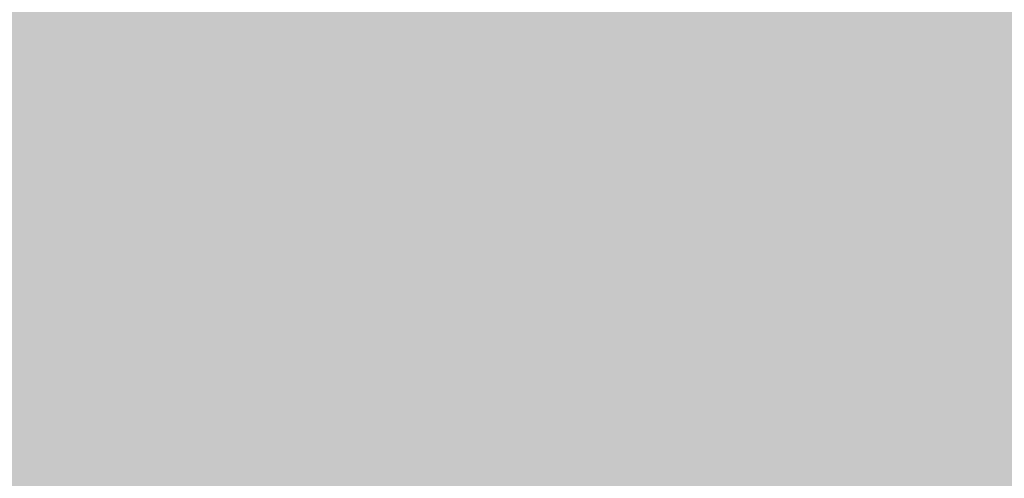
# Model space of a CAD drawing. Units: millimetres. Extents: x 0 to 2267, y 0 to 1823.
# Tile 139 of 256: x 1760 to 1802, y 1132 to 1152. Entities that reach past the tile are written whole.
import ezdxf

# ---------------------------------------------------------------- set-up
doc = ezdxf.new("R2010")
doc.units = ezdxf.units.MM
doc.header["$MEASUREMENT"] = 0
doc.layers.add('M-HATC', color=252, linetype='Continuous', lineweight=18)

msp = doc.modelspace()

# ---------------------------------------------------------------- hatches: boundary and pattern name
at = {"layer": 'M-HATC'}
h = msp.add_hatch(color=256, dxfattribs=at)
h.dxf.hatch_style = 1
h.paths.add_polyline_path([(2055.771, 1603.062), (1381.087, 1603.062), (1381.087, 1598.062), (2055.771, 1598.062)])
h.paths.add_polyline_path([(2055.771, 1598.062), (1381.087, 1598.062), (1381.087, 1593.062), (2055.771, 1593.062)])
h.paths.add_polyline_path([(2051.307, 1536.761), (1385.55, 1536.761), (1385.55, 1526.761), (1387.55, 1526.761), (1388.537, 1525.053), (1385.332, 1521.233), (1385.332, 1521.223), (2050.254, 1522.749), (2048.321, 1525.053), (2049.307, 1526.761), (2051.307, 1526.761)])
edge = h.paths.add_edge_path()
edge.add_arc((1847.535, 1379.149), 135, 222.60306, 222.89085, ccw=False)
edge.add_line((1748.166, 1287.766), (1683.092, 1287.766))
edge.add_arc((1583.724, 1379.149), 135, 317.10915, 317.39694, ccw=False)
edge.add_arc((1678.969, 1290.671), 5, 222.8909, 317.1091, ccw=False)
edge.add_arc((1774.213, 1379.149), 135, 222.60306, 222.89085, ccw=False)
edge.add_line((1674.845, 1287.766), (1609.771, 1287.766))
edge.add_arc((1510.403, 1379.149), 135, 317.10915, 317.39694, ccw=False)
edge.add_arc((1605.647, 1290.671), 5, 222.8909, 317.1091, ccw=False)
edge.add_arc((1700.892, 1379.149), 135, 222.60306, 222.89085, ccw=False)
edge.add_line((1601.524, 1287.766), (1536.45, 1287.766))
edge.add_arc((1437.081, 1379.149), 135, 317.10915, 317.39694, ccw=False)
edge.add_arc((1532.326, 1290.671), 5, 222.8909, 317.1091, ccw=False)
edge.add_arc((1627.571, 1379.149), 135, 222.60306, 222.89085, ccw=False)
edge.add_line((1528.203, 1287.766), (1505.929, 1287.766))
edge.add_spline(control_points=[(1505.929, 1287.766), (1504.262, 1287.766), (1504.262, 1282.766), (1505.929, 1282.766)], knot_values=[0, 0, 0, 0, 5, 5, 5, 5], degree=3, periodic=0)
edge.add_line((1505.929, 1282.766), (1930.929, 1282.766))
edge.add_spline(control_points=[(1930.929, 1282.766), (1932.596, 1282.766), (1932.596, 1287.766), (1930.929, 1287.766)], knot_values=[0, 0, 0, 0, 5, 5, 5, 5], degree=3, periodic=0)
edge.add_line((1930.929, 1287.766), (1903.056, 1287.766))
edge.add_arc((1803.688, 1379.149), 135, 317.10915, 317.39694, ccw=False)
edge.add_arc((1898.932, 1290.671), 5, 222.8909, 317.1091, ccw=False)
edge.add_arc((1994.177, 1379.149), 135, 222.60306, 222.89085, ccw=False)
edge.add_line((1894.809, 1287.766), (1829.735, 1287.766))
edge.add_arc((1730.366, 1379.149), 135, 317.10915, 317.39694, ccw=False)
edge.add_arc((1825.611, 1290.671), 5, 222.8909, 317.1091, ccw=False)
edge.add_arc((1920.856, 1379.149), 135, 222.60306, 222.89085, ccw=False)
edge.add_line((1821.487, 1287.766), (1756.413, 1287.766))
edge.add_arc((1657.045, 1379.149), 135, 317.10915, 317.39694, ccw=False)
edge.add_arc((1752.29, 1290.671), 5, 222.8909, 317.1091, ccw=False)
edge = h.paths.add_edge_path()
edge.add_spline(control_points=[(1843.429, 1227.247), (1845.096, 1227.247), (1845.096, 1232.247), (1843.429, 1232.247)], knot_values=[0, 0, 0, 0, 5, 5, 5, 5], degree=3, periodic=0)
edge.add_line((1843.429, 1232.247), (1593.429, 1232.247))
edge.add_spline(control_points=[(1593.429, 1232.247), (1591.762, 1232.247), (1591.762, 1227.247), (1593.429, 1227.247)], knot_values=[0, 0, 0, 0, 5, 5, 5, 5], degree=3, periodic=0)
edge.add_line((1593.429, 1227.247), (1843.429, 1227.247))
h.paths.add_polyline_path([(1905.929, 1127.417), (1530.929, 1127.417, 0.414214), (1520.929, 1117.417), (1530.929, 1117.417), (1915.929, 1117.417, 0.414214)])
edge = h.paths.add_edge_path()
edge.add_arc((1397.086, 1498.408), 12.73, 90.7821, 190.8787, ccw=False)
edge.add_line((1396.912, 1511.136), (1428.01, 1511.349))
edge.add_line((1428.01, 1511.349), (1433.01, 1511.349))
edge.add_line((1433.01, 1511.349), (1434.439, 1511.349))
edge.add_arc((1419.474, 1498.08), 20, 41.561, 74.0821)
edge.add_line((1424.959, 1517.314), (1399.935, 1517.256))
edge.add_spline(control_points=[(1399.931, 1517.256), (1399.884, 1517.213), (1399.833, 1517.169), (1399.777, 1517.124)], knot_values=[11.567499, 11.567499, 11.567499, 11.567499, 11.814249, 11.814249, 11.814249, 11.814249], degree=3, periodic=0)
edge.add_spline(control_points=[(1399.633, 1517.01), (1399.583, 1516.972), (1399.531, 1516.934), (1399.476, 1516.895)], knot_values=[11.167718, 11.167718, 11.167718, 11.167718, 11.365188, 11.365188, 11.365188, 11.365188], degree=3, periodic=0)
edge.add_spline(control_points=[(1399.34, 1516.8), (1399.151, 1516.672), (1398.938, 1516.538), (1398.704, 1516.399)], knot_values=[10.376405, 10.376405, 10.376405, 10.376405, 11.00994, 11.00994, 11.00994, 11.00994], degree=3, periodic=0)
edge.add_spline(control_points=[(1398.657, 1516.372), (1398.579, 1516.326), (1398.498, 1516.28), (1398.415, 1516.233)], knot_values=[10.125175, 10.125175, 10.125175, 10.125175, 10.334406, 10.334406, 10.334406, 10.334406], degree=3, periodic=0)
edge.add_spline(control_points=[(1398.264, 1516.149), (1398.196, 1516.111), (1398.126, 1516.073), (1398.055, 1516.035)], knot_values=[9.832246, 9.832246, 9.832246, 9.832246, 9.999658, 9.999658, 9.999658, 9.999658], degree=3, periodic=0)
edge.add_spline(control_points=[(1397.999, 1516.005), (1397.731, 1515.862), (1397.446, 1515.717), (1397.147, 1515.571)], knot_values=[9.161808, 9.161808, 9.161808, 9.161808, 9.787769, 9.787769, 9.787769, 9.787769], degree=3, periodic=0)
edge.add_spline(control_points=[(1397.147, 1515.571), (1396.842, 1515.423), (1396.522, 1515.274), (1396.191, 1515.126)], knot_values=[8.524455, 8.524455, 8.524455, 8.524455, 9.161808, 9.161808, 9.161808, 9.161808], degree=3, periodic=0)
edge.add_spline(control_points=[(1396.078, 1515.076), (1395.985, 1515.035), (1395.892, 1514.994), (1395.798, 1514.953)], knot_values=[8.275193, 8.275193, 8.275193, 8.275193, 8.451726, 8.451726, 8.451726, 8.451726], degree=3, periodic=0)
edge.add_spline(control_points=[(1395.602, 1514.869), (1395.5, 1514.826), (1395.397, 1514.782), (1395.293, 1514.739)], knot_values=[7.962917, 7.962917, 7.962917, 7.962917, 8.152764, 8.152764, 8.152764, 8.152764], degree=3, periodic=0)
edge.add_spline(control_points=[(1395.212, 1514.706), (1394.828, 1514.547), (1394.435, 1514.393), (1394.036, 1514.244)], knot_values=[7.21254, 7.21254, 7.21254, 7.21254, 7.913148, 7.913148, 7.913148, 7.913148], degree=3, periodic=0)
edge.add_spline(control_points=[(1394.036, 1514.244), (1393.708, 1514.121), (1393.375, 1514.003), (1393.043, 1513.889)], knot_values=[6.633733, 6.633733, 6.633733, 6.633733, 7.21254, 7.21254, 7.21254, 7.21254], degree=3, periodic=0)
edge.add_spline(control_points=[(1392.821, 1513.815), (1392.72, 1513.781), (1392.618, 1513.748), (1392.517, 1513.715)], knot_values=[6.328796, 6.328796, 6.328796, 6.328796, 6.505493, 6.505493, 6.505493, 6.505493], degree=3, periodic=0)
edge.add_spline(control_points=[(1392.517, 1513.715), (1392.319, 1513.652), (1392.121, 1513.59), (1391.924, 1513.531)], knot_values=[5.984605, 5.984605, 5.984605, 5.984605, 6.328796, 6.328796, 6.328796, 6.328796], degree=3, periodic=0)
edge.add_spline(control_points=[(1391.792, 1513.491), (1391.312, 1513.35), (1390.838, 1513.224), (1390.378, 1513.117)], knot_values=[5.066697, 5.066697, 5.066697, 5.066697, 5.907055, 5.907055, 5.907055, 5.907055], degree=3, periodic=0)
edge.add_spline(control_points=[(1390.378, 1513.117), (1390.18, 1513.071), (1389.984, 1513.028), (1389.791, 1512.99)], knot_values=[4.70367, 4.70367, 4.70367, 4.70367, 5.066695, 5.066695, 5.066695, 5.066695], degree=3, periodic=0)
edge.add_spline(control_points=[(1389.422, 1512.92), (1389.246, 1512.889), (1389.073, 1512.862), (1388.904, 1512.838)], knot_values=[4.130571, 4.130571, 4.130571, 4.130571, 4.469816, 4.469816, 4.469816, 4.469816], degree=3, periodic=0)
edge.add_spline(control_points=[(1388.904, 1512.838), (1388.591, 1512.795), (1388.291, 1512.764), (1388.007, 1512.749)], knot_values=[3.504031, 3.504031, 3.504031, 3.504031, 4.130571, 4.130571, 4.130571, 4.130571], degree=3, periodic=0)
edge.add_spline(control_points=[(1387.936, 1512.746), (1387.854, 1512.742), (1387.773, 1512.74), (1387.694, 1512.739)], knot_values=[3.268866, 3.268866, 3.268866, 3.268866, 3.451164, 3.451164, 3.451164, 3.451164], degree=3, periodic=0)
edge.add_spline(control_points=[(1387.335, 1512.744), (1387.208, 1512.75), (1387.085, 1512.76), (1386.967, 1512.774)], knot_values=[2.670686, 2.670686, 2.670686, 2.670686, 2.984, 2.984, 2.984, 2.984], degree=3, periodic=0)
edge.add_spline(control_points=[(1386.833, 1512.792), (1386.821, 1512.794), (1386.809, 1512.796), (1386.797, 1512.798)], knot_values=[2.516981, 2.516981, 2.516981, 2.516981, 2.549528, 2.549528, 2.549528, 2.549528], degree=3, periodic=0)
edge.add_spline(control_points=[(1386.453, 1512.873), (1386.426, 1512.881), (1386.399, 1512.889), (1386.373, 1512.897)], knot_values=[2.095869, 2.095869, 2.095869, 2.095869, 2.17941, 2.17941, 2.17941, 2.17941], degree=3, periodic=0)
edge.add_spline(control_points=[(1386.069, 1513.019), (1386.063, 1513.022), (1386.058, 1513.025), (1386.052, 1513.028)], knot_values=[1.72453, 1.72453, 1.72453, 1.72453, 1.745933, 1.745933, 1.745933, 1.745933], degree=3, periodic=0)
edge.add_arc((1399.474, 1498.08), 20, 131.8243, 180)
edge.add_arc((1630.334, 1505.548), 250.971, 181.70518, 236.42798)
edge.add_arc((1605.34, 1483.304), 218.782, 238.66083, 243.34961)
edge.add_arc((1647.091, 1510.359), 262.899, 183.12984, 237.85344, ccw=False)
h.paths.add_polyline_path([(1406.537, 1391.964, 0.149382), (1491.551, 1296.442, -0.129517)], flags=17)
edge = h.paths.add_edge_path()
edge.add_arc((2037.384, 1498.08), 20, 0, 48.2659)
edge.add_spline(control_points=[(2050.697, 1513.005), (2050.651, 1512.985), (2050.603, 1512.966), (2050.554, 1512.948)], knot_values=[1.835652, 1.835652, 1.835652, 1.835652, 2.000781, 2.000781, 2.000781, 2.000781], degree=3, periodic=0)
edge.add_spline(control_points=[(2050.462, 1512.917), (2050.479, 1512.922), (2050.496, 1512.928), (2050.513, 1512.934)], knot_values=[2.045477, 2.045477, 2.045477, 2.045477, 2.101389, 2.101389, 2.101389, 2.101389], degree=3, periodic=0)
edge.add_spline(control_points=[(2050.129, 1512.834), (2050.198, 1512.847), (2050.266, 1512.862), (2050.331, 1512.879)], knot_values=[2.237629, 2.237629, 2.237629, 2.237629, 2.435841, 2.435841, 2.435841, 2.435841], degree=3, periodic=0)
edge.add_spline(control_points=[(2050.095, 1512.828), (2050.106, 1512.83), (2050.118, 1512.832), (2050.129, 1512.834)], knot_values=[2.435841, 2.435841, 2.435841, 2.435841, 2.468321, 2.468321, 2.468321, 2.468321], degree=3, periodic=0)
edge.add_spline(control_points=[(2049.784, 1512.785), (2049.855, 1512.792), (2049.924, 1512.801), (2049.992, 1512.811)], knot_values=[2.563852, 2.563852, 2.563852, 2.563852, 2.748541, 2.748541, 2.748541, 2.748541], degree=3, periodic=0)
edge.add_spline(control_points=[(2049.405, 1512.762), (2049.536, 1512.765), (2049.663, 1512.773), (2049.784, 1512.785)], knot_values=[2.748541, 2.748541, 2.748541, 2.748541, 3.064882, 3.064882, 3.064882, 3.064882], degree=3, periodic=0)
edge.add_spline(control_points=[(2049.17, 1512.76), (2049.234, 1512.759), (2049.297, 1512.759), (2049.358, 1512.761)], knot_values=[3.102309, 3.102309, 3.102309, 3.102309, 3.2503, 3.2503, 3.2503, 3.2503], degree=3, periodic=0)
edge.add_spline(control_points=[(2048.857, 1512.769), (2048.964, 1512.764), (2049.068, 1512.761), (2049.17, 1512.76)], knot_values=[3.2503, 3.2503, 3.2503, 3.2503, 3.486069, 3.486069, 3.486069, 3.486069], degree=3, periodic=0)
edge.add_spline(control_points=[(2048.692, 1512.779), (2048.373, 1512.801), (2048.035, 1512.841), (2047.682, 1512.897)], knot_values=[3.606429, 3.606429, 3.606429, 3.606429, 4.2989, 4.2989, 4.2989, 4.2989], degree=3, periodic=0)
edge.add_spline(control_points=[(2047.682, 1512.897), (2047.546, 1512.919), (2047.408, 1512.942), (2047.268, 1512.969)], knot_values=[4.2989, 4.2989, 4.2989, 4.2989, 4.565769, 4.565769, 4.565769, 4.565769], degree=3, periodic=0)
edge.add_spline(control_points=[(2047.268, 1512.969), (2047.145, 1512.991), (2047.021, 1513.016), (2046.895, 1513.042)], knot_values=[4.565769, 4.565769, 4.565769, 4.565769, 4.799971, 4.799971, 4.799971, 4.799971], degree=3, periodic=0)
edge.add_spline(control_points=[(2046.895, 1513.042), (2046.529, 1513.119), (2046.151, 1513.209), (2045.768, 1513.311)], knot_values=[4.799971, 4.799971, 4.799971, 4.799971, 5.483718, 5.483718, 5.483718, 5.483718], degree=3, periodic=0)
edge.add_spline(control_points=[(2045.768, 1513.311), (2045.372, 1513.415), (2044.97, 1513.532), (2044.566, 1513.659)], knot_values=[5.483718, 5.483718, 5.483718, 5.483718, 6.187866, 6.187866, 6.187866, 6.187866], degree=3, periodic=0)
edge.add_spline(control_points=[(2044.566, 1513.659), (2044.415, 1513.706), (2044.263, 1513.755), (2044.112, 1513.805)], knot_values=[6.187866, 6.187866, 6.187866, 6.187866, 6.451551, 6.451551, 6.451551, 6.451551], degree=3, periodic=0)
edge.add_spline(control_points=[(2044.112, 1513.805), (2043.997, 1513.843), (2043.882, 1513.881), (2043.767, 1513.92)], knot_values=[6.451551, 6.451551, 6.451551, 6.451551, 6.651434, 6.651434, 6.651434, 6.651434], degree=3, periodic=0)
edge.add_spline(control_points=[(2043.767, 1513.92), (2043.372, 1514.055), (2042.977, 1514.198), (2042.589, 1514.346)], knot_values=[6.651434, 6.651434, 6.651434, 6.651434, 7.338879, 7.338879, 7.338879, 7.338879], degree=3, periodic=0)
edge.add_spline(control_points=[(2042.589, 1514.346), (2042.164, 1514.507), (2041.746, 1514.675), (2041.341, 1514.846)], knot_values=[7.338879, 7.338879, 7.338879, 7.338879, 8.089209, 8.089209, 8.089209, 8.089209], degree=3, periodic=0)
edge.add_spline(control_points=[(2041.341, 1514.846), (2041.103, 1514.946), (2040.869, 1515.048), (2040.64, 1515.15)], knot_values=[8.089209, 8.089209, 8.089209, 8.089209, 8.529587, 8.529587, 8.529587, 8.529587], degree=3, periodic=0)
edge.add_spline(control_points=[(2040.51, 1515.209), (2040.082, 1515.402), (2039.675, 1515.597), (2039.295, 1515.789)], knot_values=[8.613818, 8.613818, 8.613818, 8.613818, 9.44571, 9.44571, 9.44571, 9.44571], degree=3, periodic=0)
edge.add_spline(control_points=[(2039.295, 1515.789), (2039.062, 1515.907), (2038.839, 1516.025), (2038.629, 1516.14)], knot_values=[9.44571, 9.44571, 9.44571, 9.44571, 9.956404, 9.956404, 9.956404, 9.956404], degree=3, periodic=0)
edge.add_spline(control_points=[(2038.629, 1516.14), (2038.519, 1516.2), (2038.412, 1516.26), (2038.309, 1516.319)], knot_values=[9.956404, 9.956404, 9.956404, 9.956404, 10.223542, 10.223542, 10.223542, 10.223542], degree=3, periodic=0)
edge.add_spline(control_points=[(2038.309, 1516.319), (2038.214, 1516.374), (2038.122, 1516.428), (2038.033, 1516.481)], knot_values=[10.223542, 10.223542, 10.223542, 10.223542, 10.47051, 10.47051, 10.47051, 10.47051], degree=3, periodic=0)
edge.add_spline(control_points=[(2038.033, 1516.481), (2037.786, 1516.63), (2037.564, 1516.773), (2037.372, 1516.909)], knot_values=[10.47051, 10.47051, 10.47051, 10.47051, 11.15767, 11.15767, 11.15767, 11.15767], degree=3, periodic=0)
edge.add_spline(control_points=[(2037.372, 1516.909), (2037.279, 1516.975), (2037.193, 1517.04), (2037.114, 1517.102)], knot_values=[11.15767, 11.15767, 11.15767, 11.15767, 11.49227, 11.49227, 11.49227, 11.49227], degree=3, periodic=0)
edge.add_spline(control_points=[(2036.856, 1517.326), (2036.915, 1517.269), (2036.981, 1517.21), (2037.056, 1517.149)], knot_values=[11.577341, 11.577341, 11.577341, 11.577341, 11.91035, 11.91035, 11.91035, 11.91035], degree=3, periodic=0)
edge.add_spline(control_points=[(2036.807, 1517.375), (2036.823, 1517.359), (2036.839, 1517.342), (2036.856, 1517.326)], knot_values=[11.91035, 11.91035, 11.91035, 11.91035, 12.007402, 12.007402, 12.007402, 12.007402], degree=3, periodic=0)
edge.add_spline(control_points=[(2036.702, 1517.494), (2036.71, 1517.483), (2036.72, 1517.472), (2036.729, 1517.461)], knot_values=[12.184155, 12.184155, 12.184155, 12.184155, 12.255409, 12.255409, 12.255409, 12.255409], degree=3, periodic=0)
edge.add_spline(control_points=[(2036.616, 1517.621), (2036.62, 1517.613), (2036.624, 1517.606), (2036.629, 1517.598)], knot_values=[12.487913, 12.487913, 12.487913, 12.487913, 12.541035, 12.541035, 12.541035, 12.541035], degree=3, periodic=0)
edge.add_spline(control_points=[(2036.563, 1517.786), (2036.564, 1517.779), (2036.564, 1517.773), (2036.565, 1517.766)], knot_values=[12.911761, 12.911761, 12.911761, 12.911761, 12.968286, 12.968286, 12.968286, 12.968286], degree=3, periodic=0)
edge.add_spline(control_points=[(2036.617, 1517.93), (2036.612, 1517.926), (2036.609, 1517.921), (2036.605, 1517.916)], knot_values=[13.382527, 13.382527, 13.382527, 13.382527, 13.433791, 13.433791, 13.433791, 13.433791], degree=3, periodic=0)
edge.add_spline(control_points=[(2036.749, 1518.017), (2036.736, 1518.012), (2036.724, 1518.006), (2036.712, 1518)], knot_values=[13.726299, 13.726299, 13.726299, 13.726299, 13.809928, 13.809928, 13.809928, 13.809928], degree=3, periodic=0)
edge.add_spline(control_points=[(2036.86, 1518.053), (2036.839, 1518.047), (2036.818, 1518.042), (2036.799, 1518.035)], knot_values=[13.910887, 13.910887, 13.910887, 13.910887, 14.02153, 14.02153, 14.02153, 14.02153], degree=3, periodic=0)
edge.add_line((2036.964, 1518.08), (2032.384, 1518.08))
edge.add_line((2032.384, 1518.08), (2027.384, 1518.08))
edge.add_line((2027.384, 1518.08), (2022.384, 1518.08))
edge.add_line((2022.384, 1518.08), (2017.384, 1518.08))
edge.add_arc((2017.384, 1498.08), 20, 90, 138.439)
edge.add_line((2002.419, 1511.349), (2003.848, 1511.349))
edge.add_line((2003.848, 1511.349), (2008.848, 1511.349))
edge.add_line((2008.848, 1511.349), (2039.772, 1511.138))
edge.add_arc((2039.772, 1498.408), 12.73, -10.8787, 90, ccw=False)
edge.add_arc((1789.767, 1510.359), 262.899, 302.14656, 356.87016, ccw=False)
edge.add_arc((1831.518, 1483.304), 218.782, 296.65039, 301.33917)
edge.add_arc((1806.524, 1505.548), 250.971, 303.57202, 358.29482)
h.paths.add_polyline_path([(2030.321, 1391.964, -0.129517), (1945.307, 1296.442, 0.149382)], flags=17)
edge = h.paths.add_edge_path()
edge.add_spline(control_points=[(2037.246, 1518.082), (2037.29, 1518.081), (2037.336, 1518.08), (2037.384, 1518.08)], knot_values=[0.000012, 0.000012, 0.000012, 0.000012, 0.144754, 0.144754, 0.144754, 0.144754], degree=3, periodic=0)
edge.add_line((2037.336, 1518.08), (2037.01, 1518.08))
edge.add_spline(control_points=[(2037.01, 1518.08), (2036.982, 1518.077), (2036.956, 1518.073), (2036.931, 1518.068)], knot_values=[14.13465, 14.13465, 14.13465, 14.13465, 14.247197, 14.247197, 14.247197, 14.247197], degree=3, periodic=0)
edge.add_spline(control_points=[(2036.931, 1518.068), (2036.928, 1518.067), (2036.924, 1518.067), (2036.921, 1518.066)], knot_values=[14.118315, 14.118315, 14.118315, 14.118315, 14.13465, 14.13465, 14.13465, 14.13465], degree=3, periodic=0)
edge.add_spline(control_points=[(2036.921, 1518.066), (2036.912, 1518.064), (2036.903, 1518.063), (2036.895, 1518.061)], knot_values=[14.078086, 14.078086, 14.078086, 14.078086, 14.118315, 14.118315, 14.118315, 14.118315], degree=3, periodic=0)
edge.add_spline(control_points=[(2036.895, 1518.061), (2036.883, 1518.058), (2036.872, 1518.056), (2036.86, 1518.053)], knot_values=[14.02153, 14.02153, 14.02153, 14.02153, 14.078086, 14.078086, 14.078086, 14.078086], degree=3, periodic=0)
edge.add_spline(control_points=[(2036.86, 1518.053), (2036.839, 1518.047), (2036.818, 1518.042), (2036.799, 1518.035)], knot_values=[13.910887, 13.910887, 13.910887, 13.910887, 14.02153, 14.02153, 14.02153, 14.02153], degree=3, periodic=0)
edge.add_spline(control_points=[(2036.799, 1518.035), (2036.798, 1518.035), (2036.797, 1518.035), (2036.797, 1518.035)], knot_values=[13.906906, 13.906906, 13.906906, 13.906906, 13.910887, 13.910887, 13.910887, 13.910887], degree=3, periodic=0)
edge.add_spline(control_points=[(2036.797, 1518.035), (2036.788, 1518.032), (2036.78, 1518.029), (2036.772, 1518.026)], knot_values=[13.857826, 13.857826, 13.857826, 13.857826, 13.906906, 13.906906, 13.906906, 13.906906], degree=3, periodic=0)
edge.add_spline(control_points=[(2036.772, 1518.026), (2036.764, 1518.023), (2036.756, 1518.02), (2036.749, 1518.017)], knot_values=[13.809928, 13.809928, 13.809928, 13.809928, 13.857826, 13.857826, 13.857826, 13.857826], degree=3, periodic=0)
edge.add_spline(control_points=[(2036.749, 1518.017), (2036.736, 1518.012), (2036.724, 1518.006), (2036.712, 1518)], knot_values=[13.726299, 13.726299, 13.726299, 13.726299, 13.809928, 13.809928, 13.809928, 13.809928], degree=3, periodic=0)
edge.add_spline(control_points=[(2036.712, 1518), (2036.712, 1518), (2036.712, 1518), (2036.711, 1518)], knot_values=[13.723993, 13.723993, 13.723993, 13.723993, 13.726299, 13.726299, 13.726299, 13.726299], degree=3, periodic=0)
edge.add_spline(control_points=[(2036.711, 1518), (2036.706, 1517.997), (2036.701, 1517.994), (2036.696, 1517.992)], knot_values=[13.686536, 13.686536, 13.686536, 13.686536, 13.723993, 13.723993, 13.723993, 13.723993], degree=3, periodic=0)
edge.add_spline(control_points=[(2036.696, 1517.992), (2036.692, 1517.989), (2036.687, 1517.987), (2036.683, 1517.984)], knot_values=[13.651251, 13.651251, 13.651251, 13.651251, 13.686536, 13.686536, 13.686536, 13.686536], degree=3, periodic=0)
edge.add_spline(control_points=[(2036.683, 1517.984), (2036.676, 1517.98), (2036.67, 1517.976), (2036.664, 1517.971)], knot_values=[13.596804, 13.596804, 13.596804, 13.596804, 13.651251, 13.651251, 13.651251, 13.651251], degree=3, periodic=0)
edge.add_spline(control_points=[(2036.664, 1517.971), (2036.664, 1517.971), (2036.663, 1517.971), (2036.663, 1517.971)], knot_values=[13.593956, 13.593956, 13.593956, 13.593956, 13.596804, 13.596804, 13.596804, 13.596804], degree=3, periodic=0)
edge.add_spline(control_points=[(2036.663, 1517.971), (2036.66, 1517.969), (2036.658, 1517.967), (2036.655, 1517.965)], knot_values=[13.570322, 13.570322, 13.570322, 13.570322, 13.593956, 13.593956, 13.593956, 13.593956], degree=3, periodic=0)
edge.add_spline(control_points=[(2036.655, 1517.965), (2036.653, 1517.963), (2036.65, 1517.961), (2036.647, 1517.959)], knot_values=[13.545477, 13.545477, 13.545477, 13.545477, 13.570322, 13.570322, 13.570322, 13.570322], degree=3, periodic=0)
edge.add_spline(control_points=[(2036.647, 1517.959), (2036.647, 1517.959), (2036.647, 1517.959), (2036.647, 1517.959)], knot_values=[13.543931, 13.543931, 13.543931, 13.543931, 13.545477, 13.545477, 13.545477, 13.545477], degree=3, periodic=0)
edge.add_spline(control_points=[(2036.647, 1517.959), (2036.641, 1517.954), (2036.636, 1517.949), (2036.631, 1517.945)], knot_values=[13.488237, 13.488237, 13.488237, 13.488237, 13.543931, 13.543931, 13.543931, 13.543931], degree=3, periodic=0)
edge.add_spline(control_points=[(2036.631, 1517.945), (2036.628, 1517.942), (2036.626, 1517.94), (2036.623, 1517.937)], knot_values=[13.460307, 13.460307, 13.460307, 13.460307, 13.488237, 13.488237, 13.488237, 13.488237], degree=3, periodic=0)
edge.add_spline(control_points=[(2036.623, 1517.937), (2036.622, 1517.936), (2036.62, 1517.934), (2036.618, 1517.932)], knot_values=[13.439712, 13.439712, 13.439712, 13.439712, 13.460307, 13.460307, 13.460307, 13.460307], degree=3, periodic=0)
edge.add_spline(control_points=[(2036.618, 1517.932), (2036.618, 1517.931), (2036.617, 1517.931), (2036.617, 1517.93)], knot_values=[13.433791, 13.433791, 13.433791, 13.433791, 13.439712, 13.439712, 13.439712, 13.439712], degree=3, periodic=0)
edge.add_spline(control_points=[(2036.617, 1517.93), (2036.612, 1517.926), (2036.609, 1517.921), (2036.605, 1517.916)], knot_values=[13.382527, 13.382527, 13.382527, 13.382527, 13.433791, 13.433791, 13.433791, 13.433791], degree=3, periodic=0)
edge.add_spline(control_points=[(2036.605, 1517.916), (2036.603, 1517.913), (2036.6, 1517.91), (2036.598, 1517.907)], knot_values=[13.350017, 13.350017, 13.350017, 13.350017, 13.382527, 13.382527, 13.382527, 13.382527], degree=3, periodic=0)
edge.add_spline(control_points=[(2036.598, 1517.907), (2036.597, 1517.906), (2036.596, 1517.904), (2036.595, 1517.903)], knot_values=[13.333922, 13.333922, 13.333922, 13.333922, 13.350017, 13.350017, 13.350017, 13.350017], degree=3, periodic=0)
edge.add_spline(control_points=[(2036.595, 1517.903), (2036.595, 1517.902), (2036.594, 1517.901), (2036.593, 1517.9)], knot_values=[13.323828, 13.323828, 13.323828, 13.323828, 13.333922, 13.333922, 13.333922, 13.333922], degree=3, periodic=0)
edge.add_spline(control_points=[(2036.593, 1517.9), (2036.59, 1517.895), (2036.588, 1517.891), (2036.585, 1517.886)], knot_values=[13.277545, 13.277545, 13.277545, 13.277545, 13.323828, 13.323828, 13.323828, 13.323828], degree=3, periodic=0)
edge.add_spline(control_points=[(2036.585, 1517.886), (2036.584, 1517.883), (2036.582, 1517.879), (2036.58, 1517.875)], knot_values=[13.240119, 13.240119, 13.240119, 13.240119, 13.277545, 13.277545, 13.277545, 13.277545], degree=3, periodic=0)
edge.add_spline(control_points=[(2036.58, 1517.875), (2036.58, 1517.874), (2036.579, 1517.873), (2036.578, 1517.872)], knot_values=[13.228211, 13.228211, 13.228211, 13.228211, 13.240119, 13.240119, 13.240119, 13.240119], degree=3, periodic=0)
edge.add_spline(control_points=[(2036.578, 1517.872), (2036.578, 1517.87), (2036.577, 1517.869), (2036.577, 1517.868)], knot_values=[13.215717, 13.215717, 13.215717, 13.215717, 13.228211, 13.228211, 13.228211, 13.228211], degree=3, periodic=0)
edge.add_spline(control_points=[(2036.577, 1517.868), (2036.575, 1517.864), (2036.574, 1517.86), (2036.573, 1517.857)], knot_values=[13.179847, 13.179847, 13.179847, 13.179847, 13.215717, 13.215717, 13.215717, 13.215717], degree=3, periodic=0)
edge.add_spline(control_points=[(2036.573, 1517.857), (2036.571, 1517.851), (2036.57, 1517.846), (2036.569, 1517.841)], knot_values=[13.132017, 13.132017, 13.132017, 13.132017, 13.179847, 13.179847, 13.179847, 13.179847], degree=3, periodic=0)
edge.add_spline(control_points=[(2036.569, 1517.841), (2036.568, 1517.84), (2036.568, 1517.839), (2036.568, 1517.838)], knot_values=[13.122482, 13.122482, 13.122482, 13.122482, 13.132017, 13.132017, 13.132017, 13.132017], degree=3, periodic=0)
edge.add_spline(control_points=[(2036.568, 1517.838), (2036.568, 1517.836), (2036.567, 1517.835), (2036.567, 1517.833)], knot_values=[13.105592, 13.105592, 13.105592, 13.105592, 13.122482, 13.122482, 13.122482, 13.122482], degree=3, periodic=0)
edge.add_spline(control_points=[(2036.567, 1517.833), (2036.566, 1517.829), (2036.566, 1517.826), (2036.565, 1517.822)], knot_values=[13.074063, 13.074063, 13.074063, 13.074063, 13.105592, 13.105592, 13.105592, 13.105592], degree=3, periodic=0)
edge.add_spline(control_points=[(2036.565, 1517.822), (2036.565, 1517.822), (2036.565, 1517.822), (2036.565, 1517.822)], knot_values=[13.074043, 13.074043, 13.074043, 13.074043, 13.074063, 13.074063, 13.074063, 13.074063], degree=3, periodic=0)
edge.add_spline(control_points=[(2036.565, 1517.822), (2036.564, 1517.816), (2036.564, 1517.811), (2036.564, 1517.805)], knot_values=[13.021884, 13.021884, 13.021884, 13.021884, 13.074043, 13.074043, 13.074043, 13.074043], degree=3, periodic=0)
edge.add_spline(control_points=[(2036.564, 1517.805), (2036.564, 1517.804), (2036.564, 1517.803), (2036.564, 1517.803)], knot_values=[13.01674, 13.01674, 13.01674, 13.01674, 13.021884, 13.021884, 13.021884, 13.021884], degree=3, periodic=0)
edge.add_spline(control_points=[(2036.564, 1517.803), (2036.563, 1517.801), (2036.563, 1517.798), (2036.563, 1517.796)], knot_values=[12.996438, 12.996438, 12.996438, 12.996438, 13.01674, 13.01674, 13.01674, 13.01674], degree=3, periodic=0)
edge.add_spline(control_points=[(2036.563, 1517.796), (2036.563, 1517.793), (2036.563, 1517.789), (2036.563, 1517.786)], knot_values=[12.968286, 12.968286, 12.968286, 12.968286, 12.996438, 12.996438, 12.996438, 12.996438], degree=3, periodic=0)
edge.add_spline(control_points=[(2036.563, 1517.786), (2036.564, 1517.779), (2036.564, 1517.773), (2036.565, 1517.766)], knot_values=[12.911761, 12.911761, 12.911761, 12.911761, 12.968286, 12.968286, 12.968286, 12.968286], degree=3, periodic=0)
edge.add_spline(control_points=[(2036.565, 1517.766), (2036.565, 1517.766), (2036.565, 1517.766), (2036.565, 1517.766)], knot_values=[12.911017, 12.911017, 12.911017, 12.911017, 12.911761, 12.911761, 12.911761, 12.911761], degree=3, periodic=0)
edge.add_spline(control_points=[(2036.565, 1517.766), (2036.565, 1517.762), (2036.566, 1517.759), (2036.566, 1517.756)], knot_values=[12.88528, 12.88528, 12.88528, 12.88528, 12.911017, 12.911017, 12.911017, 12.911017], degree=3, periodic=0)
edge.add_spline(control_points=[(2036.566, 1517.756), (2036.567, 1517.753), (2036.567, 1517.751), (2036.568, 1517.748)], knot_values=[12.862519, 12.862519, 12.862519, 12.862519, 12.88528, 12.88528, 12.88528, 12.88528], degree=3, periodic=0)
edge.add_spline(control_points=[(2036.568, 1517.748), (2036.568, 1517.747), (2036.568, 1517.747), (2036.568, 1517.746)], knot_values=[12.858885, 12.858885, 12.858885, 12.858885, 12.862519, 12.862519, 12.862519, 12.862519], degree=3, periodic=0)
edge.add_spline(control_points=[(2036.568, 1517.746), (2036.569, 1517.74), (2036.571, 1517.733), (2036.572, 1517.726)], knot_values=[12.8053, 12.8053, 12.8053, 12.8053, 12.858885, 12.858885, 12.858885, 12.858885], degree=3, periodic=0)
edge.add_spline(control_points=[(2036.572, 1517.726), (2036.573, 1517.723), (2036.574, 1517.719), (2036.576, 1517.715)], knot_values=[12.775176, 12.775176, 12.775176, 12.775176, 12.8053, 12.8053, 12.8053, 12.8053], degree=3, periodic=0)
edge.add_spline(control_points=[(2036.576, 1517.715), (2036.576, 1517.713), (2036.577, 1517.71), (2036.578, 1517.708)], knot_values=[12.756759, 12.756759, 12.756759, 12.756759, 12.775176, 12.775176, 12.775176, 12.775176], degree=3, periodic=0)
edge.add_spline(control_points=[(2036.578, 1517.708), (2036.578, 1517.707), (2036.578, 1517.706), (2036.579, 1517.705)], knot_values=[12.748742, 12.748742, 12.748742, 12.748742, 12.756759, 12.756759, 12.756759, 12.756759], degree=3, periodic=0)
edge.add_spline(control_points=[(2036.579, 1517.705), (2036.581, 1517.698), (2036.583, 1517.692), (2036.586, 1517.685)], knot_values=[12.69959, 12.69959, 12.69959, 12.69959, 12.748742, 12.748742, 12.748742, 12.748742], degree=3, periodic=0)
edge.add_spline(control_points=[(2036.586, 1517.685), (2036.588, 1517.68), (2036.59, 1517.675), (2036.592, 1517.669)], knot_values=[12.659038, 12.659038, 12.659038, 12.659038, 12.69959, 12.69959, 12.69959, 12.69959], degree=3, periodic=0)
edge.add_spline(control_points=[(2036.592, 1517.669), (2036.594, 1517.665), (2036.596, 1517.66), (2036.598, 1517.656)], knot_values=[12.626806, 12.626806, 12.626806, 12.626806, 12.659038, 12.659038, 12.659038, 12.659038], degree=3, periodic=0)
edge.add_spline(control_points=[(2036.598, 1517.656), (2036.598, 1517.655), (2036.599, 1517.654), (2036.599, 1517.653)], knot_values=[12.619394, 12.619394, 12.619394, 12.619394, 12.626806, 12.626806, 12.626806, 12.626806], degree=3, periodic=0)
edge.add_spline(control_points=[(2036.599, 1517.653), (2036.604, 1517.642), (2036.61, 1517.632), (2036.616, 1517.621)], knot_values=[12.541039, 12.541039, 12.541039, 12.541039, 12.619394, 12.619394, 12.619394, 12.619394], degree=3, periodic=0)
edge.add_spline(control_points=[(2036.616, 1517.621), (2036.616, 1517.621), (2036.616, 1517.621), (2036.616, 1517.621)], knot_values=[12.541035, 12.541035, 12.541035, 12.541035, 12.541039, 12.541039, 12.541039, 12.541039], degree=3, periodic=0)
edge.add_spline(control_points=[(2036.616, 1517.621), (2036.62, 1517.613), (2036.624, 1517.606), (2036.629, 1517.598)], knot_values=[12.487913, 12.487913, 12.487913, 12.487913, 12.541035, 12.541035, 12.541035, 12.541035], degree=3, periodic=0)
edge.add_spline(control_points=[(2036.629, 1517.598), (2036.633, 1517.592), (2036.637, 1517.585), (2036.641, 1517.579)], knot_values=[12.443982, 12.443982, 12.443982, 12.443982, 12.487913, 12.487913, 12.487913, 12.487913], degree=3, periodic=0)
edge.add_spline(control_points=[(2036.641, 1517.579), (2036.641, 1517.578), (2036.642, 1517.576), (2036.643, 1517.575)], knot_values=[12.434996, 12.434996, 12.434996, 12.434996, 12.443982, 12.443982, 12.443982, 12.443982], degree=3, periodic=0)
edge.add_spline(control_points=[(2036.643, 1517.575), (2036.653, 1517.56), (2036.664, 1517.544), (2036.676, 1517.528)], knot_values=[12.329647, 12.329647, 12.329647, 12.329647, 12.434996, 12.434996, 12.434996, 12.434996], degree=3, periodic=0)
edge.add_spline(control_points=[(2036.676, 1517.528), (2036.684, 1517.517), (2036.693, 1517.505), (2036.702, 1517.494)], knot_values=[12.255409, 12.255409, 12.255409, 12.255409, 12.329647, 12.329647, 12.329647, 12.329647], degree=3, periodic=0)
edge.add_spline(control_points=[(2036.702, 1517.494), (2036.71, 1517.483), (2036.72, 1517.472), (2036.729, 1517.461)], knot_values=[12.184155, 12.184155, 12.184155, 12.184155, 12.255409, 12.255409, 12.255409, 12.255409], degree=3, periodic=0)
edge.add_spline(control_points=[(2036.729, 1517.461), (2036.744, 1517.444), (2036.759, 1517.426), (2036.775, 1517.409)], knot_values=[12.075961, 12.075961, 12.075961, 12.075961, 12.184155, 12.184155, 12.184155, 12.184155], degree=3, periodic=0)
edge.add_spline(control_points=[(2036.775, 1517.409), (2036.776, 1517.407), (2036.777, 1517.406), (2036.778, 1517.405)], knot_values=[12.069502, 12.069502, 12.069502, 12.069502, 12.075961, 12.075961, 12.075961, 12.075961], degree=3, periodic=0)
edge.add_spline(control_points=[(2036.778, 1517.405), (2036.788, 1517.395), (2036.797, 1517.385), (2036.807, 1517.375)], knot_values=[12.007402, 12.007402, 12.007402, 12.007402, 12.069502, 12.069502, 12.069502, 12.069502], degree=3, periodic=0)
edge.add_spline(control_points=[(2036.807, 1517.375), (2036.823, 1517.359), (2036.839, 1517.342), (2036.856, 1517.326)], knot_values=[11.91035, 11.91035, 11.91035, 11.91035, 12.007402, 12.007402, 12.007402, 12.007402], degree=3, periodic=0)
edge.add_spline(control_points=[(2036.856, 1517.326), (2036.915, 1517.269), (2036.981, 1517.21), (2037.056, 1517.149)], knot_values=[11.577341, 11.577341, 11.577341, 11.577341, 11.91035, 11.91035, 11.91035, 11.91035], degree=3, periodic=0)
edge.add_spline(control_points=[(2037.056, 1517.149), (2037.075, 1517.134), (2037.094, 1517.118), (2037.114, 1517.102)], knot_values=[11.49227, 11.49227, 11.49227, 11.49227, 11.577341, 11.577341, 11.577341, 11.577341], degree=3, periodic=0)
edge.add_spline(control_points=[(2037.114, 1517.102), (2037.193, 1517.04), (2037.279, 1516.975), (2037.372, 1516.909)], knot_values=[11.15767, 11.15767, 11.15767, 11.15767, 11.49227, 11.49227, 11.49227, 11.49227], degree=3, periodic=0)
edge.add_spline(control_points=[(2037.372, 1516.909), (2037.564, 1516.773), (2037.786, 1516.63), (2038.033, 1516.481)], knot_values=[10.47051, 10.47051, 10.47051, 10.47051, 11.15767, 11.15767, 11.15767, 11.15767], degree=3, periodic=0)
edge.add_spline(control_points=[(2038.033, 1516.481), (2038.122, 1516.428), (2038.214, 1516.374), (2038.309, 1516.319)], knot_values=[10.223542, 10.223542, 10.223542, 10.223542, 10.47051, 10.47051, 10.47051, 10.47051], degree=3, periodic=0)
edge.add_spline(control_points=[(2038.309, 1516.319), (2038.412, 1516.26), (2038.519, 1516.2), (2038.629, 1516.14)], knot_values=[9.956404, 9.956404, 9.956404, 9.956404, 10.223542, 10.223542, 10.223542, 10.223542], degree=3, periodic=0)
edge.add_spline(control_points=[(2038.629, 1516.14), (2038.839, 1516.025), (2039.062, 1515.907), (2039.295, 1515.789)], knot_values=[9.44571, 9.44571, 9.44571, 9.44571, 9.956404, 9.956404, 9.956404, 9.956404], degree=3, periodic=0)
edge.add_spline(control_points=[(2039.295, 1515.789), (2039.675, 1515.597), (2040.082, 1515.402), (2040.51, 1515.209)], knot_values=[8.613818, 8.613818, 8.613818, 8.613818, 9.44571, 9.44571, 9.44571, 9.44571], degree=3, periodic=0)
edge.add_spline(control_points=[(2040.51, 1515.209), (2040.553, 1515.189), (2040.597, 1515.17), (2040.64, 1515.15)], knot_values=[8.529587, 8.529587, 8.529587, 8.529587, 8.613818, 8.613818, 8.613818, 8.613818], degree=3, periodic=0)
edge.add_spline(control_points=[(2040.64, 1515.15), (2040.869, 1515.048), (2041.103, 1514.946), (2041.341, 1514.846)], knot_values=[8.089209, 8.089209, 8.089209, 8.089209, 8.529587, 8.529587, 8.529587, 8.529587], degree=3, periodic=0)
edge.add_spline(control_points=[(2041.341, 1514.846), (2041.746, 1514.675), (2042.164, 1514.507), (2042.589, 1514.346)], knot_values=[7.338879, 7.338879, 7.338879, 7.338879, 8.089209, 8.089209, 8.089209, 8.089209], degree=3, periodic=0)
edge.add_spline(control_points=[(2042.589, 1514.346), (2042.977, 1514.198), (2043.372, 1514.055), (2043.767, 1513.92)], knot_values=[6.651434, 6.651434, 6.651434, 6.651434, 7.338879, 7.338879, 7.338879, 7.338879], degree=3, periodic=0)
edge.add_spline(control_points=[(2043.767, 1513.92), (2043.882, 1513.881), (2043.997, 1513.843), (2044.112, 1513.805)], knot_values=[6.451551, 6.451551, 6.451551, 6.451551, 6.651434, 6.651434, 6.651434, 6.651434], degree=3, periodic=0)
edge.add_spline(control_points=[(2044.112, 1513.805), (2044.263, 1513.755), (2044.415, 1513.706), (2044.566, 1513.659)], knot_values=[6.187866, 6.187866, 6.187866, 6.187866, 6.451551, 6.451551, 6.451551, 6.451551], degree=3, periodic=0)
edge.add_spline(control_points=[(2044.566, 1513.659), (2044.97, 1513.532), (2045.372, 1513.415), (2045.768, 1513.311)], knot_values=[5.483718, 5.483718, 5.483718, 5.483718, 6.187866, 6.187866, 6.187866, 6.187866], degree=3, periodic=0)
edge.add_spline(control_points=[(2045.768, 1513.311), (2046.151, 1513.209), (2046.529, 1513.119), (2046.895, 1513.042)], knot_values=[4.799971, 4.799971, 4.799971, 4.799971, 5.483718, 5.483718, 5.483718, 5.483718], degree=3, periodic=0)
edge.add_spline(control_points=[(2046.895, 1513.042), (2047.021, 1513.016), (2047.145, 1512.991), (2047.268, 1512.969)], knot_values=[4.565769, 4.565769, 4.565769, 4.565769, 4.799971, 4.799971, 4.799971, 4.799971], degree=3, periodic=0)
edge.add_spline(control_points=[(2047.268, 1512.969), (2047.408, 1512.942), (2047.546, 1512.919), (2047.682, 1512.897)], knot_values=[4.2989, 4.2989, 4.2989, 4.2989, 4.565769, 4.565769, 4.565769, 4.565769], degree=3, periodic=0)
edge.add_spline(control_points=[(2047.682, 1512.897), (2048.035, 1512.841), (2048.373, 1512.801), (2048.692, 1512.779)], knot_values=[3.606429, 3.606429, 3.606429, 3.606429, 4.2989, 4.2989, 4.2989, 4.2989], degree=3, periodic=0)
edge.add_spline(control_points=[(2048.692, 1512.779), (2048.748, 1512.775), (2048.803, 1512.772), (2048.857, 1512.769)], knot_values=[3.486069, 3.486069, 3.486069, 3.486069, 3.606429, 3.606429, 3.606429, 3.606429], degree=3, periodic=0)
edge.add_spline(control_points=[(2048.857, 1512.769), (2048.964, 1512.764), (2049.068, 1512.761), (2049.17, 1512.76)], knot_values=[3.2503, 3.2503, 3.2503, 3.2503, 3.486069, 3.486069, 3.486069, 3.486069], degree=3, periodic=0)
edge.add_spline(control_points=[(2049.17, 1512.76), (2049.234, 1512.759), (2049.297, 1512.759), (2049.358, 1512.761)], knot_values=[3.102309, 3.102309, 3.102309, 3.102309, 3.2503, 3.2503, 3.2503, 3.2503], degree=3, periodic=0)
edge.add_spline(control_points=[(2049.358, 1512.761), (2049.374, 1512.761), (2049.39, 1512.761), (2049.405, 1512.762)], knot_values=[3.064882, 3.064882, 3.064882, 3.064882, 3.102309, 3.102309, 3.102309, 3.102309], degree=3, periodic=0)
edge.add_spline(control_points=[(2049.405, 1512.762), (2049.536, 1512.765), (2049.663, 1512.773), (2049.784, 1512.785)], knot_values=[2.748541, 2.748541, 2.748541, 2.748541, 3.064882, 3.064882, 3.064882, 3.064882], degree=3, periodic=0)
edge.add_spline(control_points=[(2049.784, 1512.785), (2049.855, 1512.792), (2049.924, 1512.801), (2049.992, 1512.811)], knot_values=[2.563852, 2.563852, 2.563852, 2.563852, 2.748541, 2.748541, 2.748541, 2.748541], degree=3, periodic=0)
edge.add_spline(control_points=[(2049.992, 1512.811), (2050.026, 1512.816), (2050.061, 1512.822), (2050.095, 1512.828)], knot_values=[2.468321, 2.468321, 2.468321, 2.468321, 2.563852, 2.563852, 2.563852, 2.563852], degree=3, periodic=0)
edge.add_spline(control_points=[(2050.095, 1512.828), (2050.106, 1512.83), (2050.118, 1512.832), (2050.129, 1512.834)], knot_values=[2.435841, 2.435841, 2.435841, 2.435841, 2.468321, 2.468321, 2.468321, 2.468321], degree=3, periodic=0)
edge.add_spline(control_points=[(2050.129, 1512.834), (2050.198, 1512.847), (2050.266, 1512.862), (2050.331, 1512.879)], knot_values=[2.237629, 2.237629, 2.237629, 2.237629, 2.435841, 2.435841, 2.435841, 2.435841], degree=3, periodic=0)
edge.add_spline(control_points=[(2050.331, 1512.879), (2050.375, 1512.891), (2050.419, 1512.903), (2050.462, 1512.917)], knot_values=[2.101389, 2.101389, 2.101389, 2.101389, 2.237629, 2.237629, 2.237629, 2.237629], degree=3, periodic=0)
edge.add_spline(control_points=[(2050.462, 1512.917), (2050.479, 1512.922), (2050.496, 1512.928), (2050.513, 1512.934)], knot_values=[2.045477, 2.045477, 2.045477, 2.045477, 2.101389, 2.101389, 2.101389, 2.101389], degree=3, periodic=0)
edge.add_spline(control_points=[(2050.513, 1512.934), (2050.527, 1512.938), (2050.54, 1512.943), (2050.554, 1512.948)], knot_values=[2.000781, 2.000781, 2.000781, 2.000781, 2.045477, 2.045477, 2.045477, 2.045477], degree=3, periodic=0)
edge.add_spline(control_points=[(2050.554, 1512.948), (2050.603, 1512.966), (2050.651, 1512.985), (2050.697, 1513.005)], knot_values=[1.835652, 1.835652, 1.835652, 1.835652, 2.000781, 2.000781, 2.000781, 2.000781], degree=3, periodic=0)
edge.add_arc((2037.384, 1498.08), 20, 48.2659, 90.1299)
edge = h.paths.add_edge_path(flags=16)
edge.add_spline(control_points=[(1386.139, 1512.986), (1388.92, 1511.739), (1398.039, 1515.519), (1399.931, 1517.256)], knot_values=[1.831046, 1.831046, 1.831046, 1.831046, 11.814249, 11.814249, 11.814249, 11.814249], degree=3, periodic=0)
edge.add_line((1399.931, 1517.256), (1393.743, 1517.242))
edge.add_arc((1399.474, 1498.08), 20, 106.6501, 131.8173)
h = msp.add_hatch(color=256, dxfattribs=at)
h.dxf.hatch_style = 1
h.paths.add_polyline_path([(2042.889, 1580.18), (2055.771, 1593.062), (1381.087, 1593.062), (1393.969, 1580.18), (1374.086, 1560.296), (2062.772, 1560.296)])
h.paths.add_polyline_path([(1843.429, 1201.33), (1843.429, 1227.247), (1593.429, 1227.247), (1593.429, 1201.33, -0.228274), (1574.599, 1162.235), (1530.929, 1127.417), (1905.929, 1127.417), (1862.259, 1162.235, -0.228274)])

doc.saveas('drawing.dxf')
